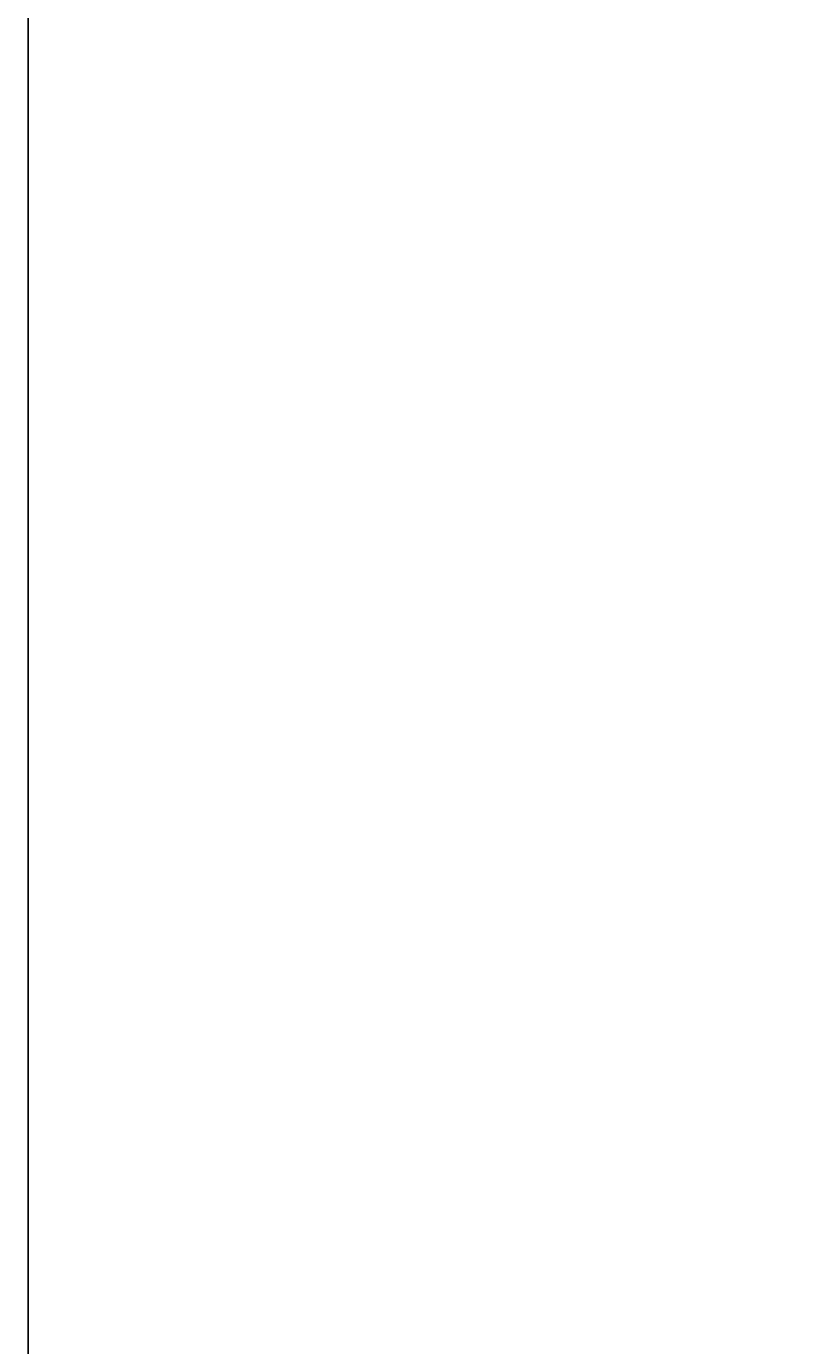
# Model space of a CAD drawing. Units: inches. Extents: x 3731 to 4318, y 1310 to 2388.
# Tile 2 of 57: x 3731 to 3828, y 1393 to 1554. Entities that reach past the tile are written whole.
import ezdxf

# ---------------------------------------------------------------- set-up
doc = ezdxf.new("R2010")
doc.units = ezdxf.units.IN
doc.layers.add('A-ANNO-DIMS', color=2, linetype='Continuous', lineweight=18)
doc.styles.get("Standard").update_dxf_attribs({"font": 'arial.ttf'})
doc.dimstyles.get("Standard").update_dxf_attribs({"dimtxt": 0.18, "dimasz": 0.18, "dimexe": 0.18, "dimexo": 0.0625, "dimgap": 0.09, "dimtad": 0, "dimtih": 1, "dimtoh": 1, "dimdec": 4, "dimzin": 0, "dimdsep": 46, "dimtxsty": 'Standard', "dimcen": 0.09, "dimadec": 0, "dimazin": 0, "dimtfac": 1, "dimtdec": 4, "dimtofl": 0, "dimtmove": 0, "dimatfit": 3, "dimfxl": 1, "dimtolj": 1, "dimtzin": 0, "dimarcsym": 0})

# ---------------------------------------------------------------- blocks, each defined once
blk = doc.blocks.new('*D33')
at = {"layer": 'A-ANNO-DIMS', "color": 0, "lineweight": -2, "transparency": 16777216}
for p, q in [((3835.15, 2338.38), (3731.41, 2338.38)), ((3731.59, 2338.2), (3731.59, 1849.06)), ((3731.59, 1359.56), (3731.59, 1848.7)), ((3835.15, 1359.38), (3731.41, 1359.38))]:
    blk.add_line(p, q, dxfattribs=at)
at = {"layer": 'A-ANNO-DIMS', "color": 0, "transparency": 16777216}
for points in [[(3731.56, 2338.2), (3731.62, 2338.2), (3731.59, 2338.38)], [(3731.56, 1359.56), (3731.62, 1359.56), (3731.59, 1359.38)]]:
    blk.add_solid(points, dxfattribs=at)
at = {"layer": 'Defpoints', "color": 0, "transparency": 16777216}
for p in [(3731.59, 2338.38), (3835.21, 2338.38), (3835.21, 1359.38)]:
    blk.add_point(p, dxfattribs=at)
at = {"layer": 'A-ANNO-DIMS', "color": 0, "transparency": 16777216, "insert": (3731.59, 1848.88), "char_height": 0.18, "attachment_point": 5}
blk.add_mtext('\\A1;979', dxfattribs=at)

msp = doc.modelspace()

# ---------------------------------------------------------------- dimensions: what is measured, and where the dimension line sits
at = {"layer": 'A-ANNO-DIMS'}
dim = msp.add_linear_dim(base=(3731.59, 2338.38), p1=(3835.21, 1359.38), p2=(3835.21, 2338.38), angle=90, dimstyle='Standard', override={"dimdec": 0, "dimlfac": 1, "dimrnd": 0, "dimzin": 0, "dimdsep": 46, "dimlunit": 2}, dxfattribs=at)
dim.commit()
dim.dimension.update_dxf_attribs({"geometry": '*D33', "text_midpoint": (3731.59, 1848.88)})

doc.saveas('drawing.dxf')
